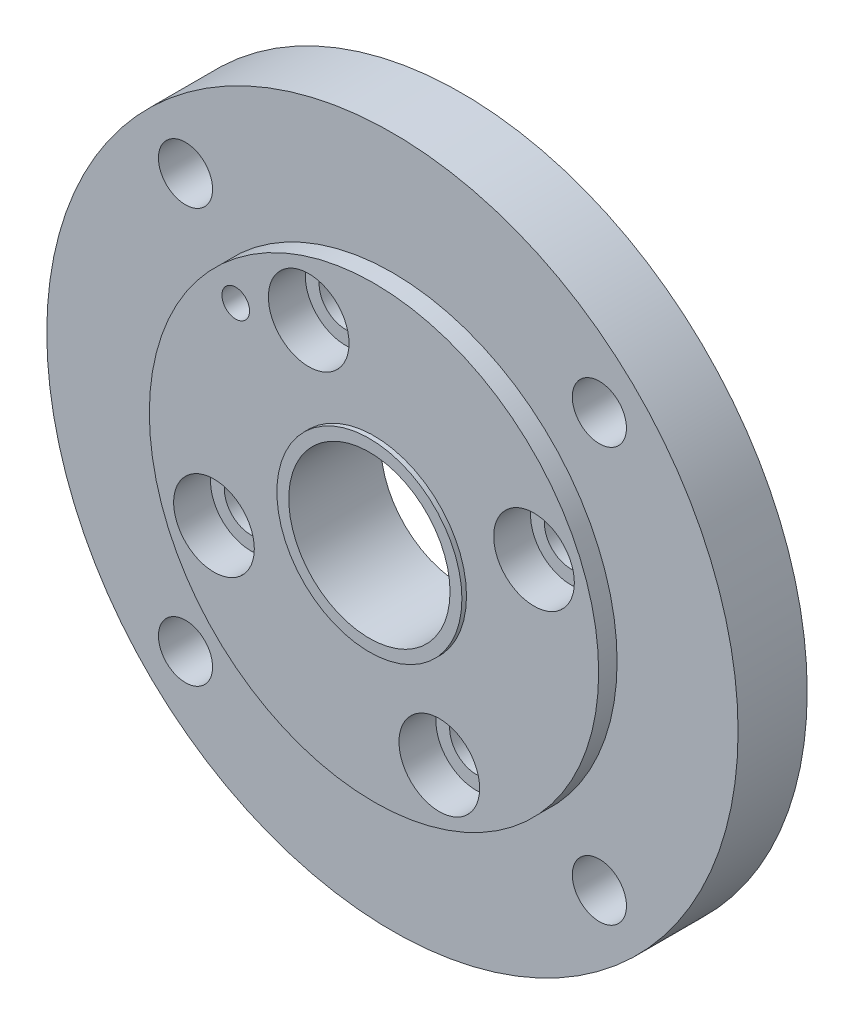
ISO-10303-21;
HEADER;
FILE_DESCRIPTION(('STEP AP214'),'2;1');
FILE_NAME('part.step','',(''),(''),'','','');
FILE_SCHEMA(('AUTOMOTIVE_DESIGN { 1 0 10303 214 1 1 1 1 }'));
ENDSEC;
DATA;
#1=APPLICATION_CONTEXT('core data for automotive mechanical design processes');
#2=APPLICATION_PROTOCOL_DEFINITION('international standard','automotive_design',2000,#1);
#3=PRODUCT_CONTEXT('',#1,'mechanical');
#4=PRODUCT('Part','Part','',(#3));
#5=PRODUCT_RELATED_PRODUCT_CATEGORY('part','',(#4));
#6=PRODUCT_DEFINITION_FORMATION('','',#4);
#7=PRODUCT_DEFINITION_CONTEXT('part definition',#1,'design');
#8=PRODUCT_DEFINITION('design','',#6,#7);
#9=PRODUCT_DEFINITION_SHAPE('','',#8);
#10=(LENGTH_UNIT() NAMED_UNIT(*) SI_UNIT(.MILLI.,.METRE.));
#11=(NAMED_UNIT(*) PLANE_ANGLE_UNIT() SI_UNIT($,.RADIAN.));
#12=(NAMED_UNIT(*) SI_UNIT($,.STERADIAN.) SOLID_ANGLE_UNIT());
#13=UNCERTAINTY_MEASURE_WITH_UNIT(LENGTH_MEASURE(1.E-05),#10,'distance_accuracy_value','');
#14=(GEOMETRIC_REPRESENTATION_CONTEXT(3) GLOBAL_UNCERTAINTY_ASSIGNED_CONTEXT((#13)) GLOBAL_UNIT_ASSIGNED_CONTEXT((#10,
#11,#12)) REPRESENTATION_CONTEXT('',''));
#15=CARTESIAN_POINT('',(0.,0.,0.));
#16=DIRECTION('',(0.,0.,1.));
#17=DIRECTION('',(1.,0.,0.));
#18=AXIS2_PLACEMENT_3D('',#15,#16,#17);
#19=CARTESIAN_POINT('',(0.,0.,30.));
#20=DIRECTION('',(0.,0.,-1.));
#21=DIRECTION('',(-1.,0.,0.));
#22=AXIS2_PLACEMENT_3D('',#19,#20,#21);
#23=CYLINDRICAL_SURFACE('',#22,150.);
#24=CARTESIAN_POINT('',(0.,0.,30.));
#25=DIRECTION('',(0.,0.,1.));
#26=DIRECTION('',(1.,0.,0.));
#27=AXIS2_PLACEMENT_3D('',#24,#25,#26);
#28=CIRCLE('',#27,150.);
#29=CARTESIAN_POINT('',(150.,0.,30.));
#30=VERTEX_POINT('',#29);
#31=EDGE_CURVE('E54',#30,#30,#28,.T.);
#32=ORIENTED_EDGE('',*,*,#31,.F.);
#33=EDGE_LOOP('',(#32));
#34=FACE_BOUND('',#33,.T.);
#35=CARTESIAN_POINT('',(0.,0.,0.));
#36=DIRECTION('',(0.,0.,1.));
#37=DIRECTION('',(1.,0.,0.));
#38=AXIS2_PLACEMENT_3D('',#35,#36,#37);
#39=CIRCLE('',#38,150.);
#40=CARTESIAN_POINT('',(150.,0.,0.));
#41=VERTEX_POINT('',#40);
#42=EDGE_CURVE('E65',#41,#41,#39,.T.);
#43=ORIENTED_EDGE('',*,*,#42,.T.);
#44=EDGE_LOOP('',(#43));
#45=FACE_BOUND('',#44,.T.);
#46=ADVANCED_FACE('F43',(#34,#45),#23,.T.);
#47=CARTESIAN_POINT('',(0.,0.,30.));
#48=DIRECTION('',(0.,0.,1.));
#49=DIRECTION('',(1.,0.,0.));
#50=AXIS2_PLACEMENT_3D('',#47,#48,#49);
#51=PLANE('',#50);
#52=CARTESIAN_POINT('',(-89.8025612106864,-89.8025612106967,30.));
#53=DIRECTION('',(0.,0.,1.));
#54=DIRECTION('',(1.,0.,0.));
#55=AXIS2_PLACEMENT_3D('',#52,#53,#54);
#56=CIRCLE('',#55,11.7500000000037);
#57=CARTESIAN_POINT('',(-78.0525612106827,-89.8025612106967,30.));
#58=VERTEX_POINT('',#57);
#59=EDGE_CURVE('E118',#58,#58,#56,.T.);
#60=ORIENTED_EDGE('',*,*,#59,.F.);
#61=EDGE_LOOP('',(#60));
#62=FACE_BOUND('',#61,.T.);
#63=CARTESIAN_POINT('',(89.8025612106966,-89.8025612106914,30.));
#64=DIRECTION('',(0.,0.,1.));
#65=DIRECTION('',(1.,0.,0.));
#66=AXIS2_PLACEMENT_3D('',#63,#64,#65);
#67=CIRCLE('',#66,11.7499999999988);
#68=CARTESIAN_POINT('',(101.552561210695,-89.8025612106914,30.));
#69=VERTEX_POINT('',#68);
#70=EDGE_CURVE('E120',#69,#69,#67,.T.);
#71=ORIENTED_EDGE('',*,*,#70,.F.);
#72=EDGE_LOOP('',(#71));
#73=FACE_BOUND('',#72,.T.);
#74=CARTESIAN_POINT('',(89.8025612106914,89.8025612106917,30.));
#75=DIRECTION('',(0.,0.,1.));
#76=DIRECTION('',(1.,0.,0.));
#77=AXIS2_PLACEMENT_3D('',#74,#75,#76);
#78=CIRCLE('',#77,11.75);
#79=CARTESIAN_POINT('',(101.552561210691,89.8025612106917,30.));
#80=VERTEX_POINT('',#79);
#81=EDGE_CURVE('E113',#80,#80,#78,.T.);
#82=ORIENTED_EDGE('',*,*,#81,.F.);
#83=EDGE_LOOP('',(#82));
#84=FACE_BOUND('',#83,.T.);
#85=CARTESIAN_POINT('',(-89.8025612106917,89.8025612106864,30.));
#86=DIRECTION('',(0.,0.,1.));
#87=DIRECTION('',(1.,0.,0.));
#88=AXIS2_PLACEMENT_3D('',#85,#86,#87);
#89=CIRCLE('',#88,11.7500000000053);
#90=CARTESIAN_POINT('',(-78.0525612106864,89.8025612106864,30.));
#91=VERTEX_POINT('',#90);
#92=EDGE_CURVE('E75',#91,#91,#89,.T.);
#93=ORIENTED_EDGE('',*,*,#92,.F.);
#94=EDGE_LOOP('',(#93));
#95=FACE_BOUND('',#94,.T.);
#96=CARTESIAN_POINT('',(0.,0.,30.));
#97=DIRECTION('',(0.,0.,1.));
#98=DIRECTION('',(1.,0.,0.));
#99=AXIS2_PLACEMENT_3D('',#96,#97,#98);
#100=CIRCLE('',#99,97.5);
#101=CARTESIAN_POINT('',(97.5,0.,30.));
#102=VERTEX_POINT('',#101);
#103=EDGE_CURVE('E49',#102,#102,#100,.T.);
#104=ORIENTED_EDGE('',*,*,#103,.F.);
#105=EDGE_LOOP('',(#104));
#106=FACE_BOUND('',#105,.T.);
#107=ORIENTED_EDGE('',*,*,#31,.T.);
#108=EDGE_LOOP('',(#107));
#109=FACE_BOUND('',#108,.T.);
#110=ADVANCED_FACE('F148',(#62,#73,#84,#95,#106,#109),#51,.T.);
#111=CARTESIAN_POINT('',(0.,0.,0.));
#112=DIRECTION('',(0.,0.,1.));
#113=DIRECTION('',(1.,0.,0.));
#114=AXIS2_PLACEMENT_3D('',#111,#112,#113);
#115=PLANE('',#114);
#116=CARTESIAN_POINT('',(0.,0.,0.));
#117=DIRECTION('',(0.,0.,1.));
#118=DIRECTION('',(1.,0.,0.));
#119=AXIS2_PLACEMENT_3D('',#116,#117,#118);
#120=CIRCLE('',#119,35.);
#121=CARTESIAN_POINT('',(35.,0.,0.));
#122=VERTEX_POINT('',#121);
#123=EDGE_CURVE('E170',#122,#122,#120,.T.);
#124=ORIENTED_EDGE('',*,*,#123,.T.);
#125=EDGE_LOOP('',(#124));
#126=FACE_BOUND('',#125,.T.);
#127=CARTESIAN_POINT('',(-28.3380590113851,69.4402938607496,0.));
#128=DIRECTION('',(0.,0.,1.));
#129=DIRECTION('',(1.,0.,0.));
#130=AXIS2_PLACEMENT_3D('',#127,#128,#129);
#131=CIRCLE('',#130,11.5);
#132=CARTESIAN_POINT('',(-16.8380590113851,69.4402938607496,0.));
#133=VERTEX_POINT('',#132);
#134=EDGE_CURVE('E46',#133,#133,#131,.T.);
#135=ORIENTED_EDGE('',*,*,#134,.T.);
#136=EDGE_LOOP('',(#135));
#137=FACE_BOUND('',#136,.T.);
#138=CARTESIAN_POINT('',(69.4402938607507,28.3380590113878,0.));
#139=DIRECTION('',(0.,0.,1.));
#140=DIRECTION('',(1.,0.,0.));
#141=AXIS2_PLACEMENT_3D('',#138,#139,#140);
#142=CIRCLE('',#141,11.5000000000026);
#143=CARTESIAN_POINT('',(80.9402938607533,28.3380590113878,0.));
#144=VERTEX_POINT('',#143);
#145=EDGE_CURVE('E78',#144,#144,#142,.T.);
#146=ORIENTED_EDGE('',*,*,#145,.T.);
#147=EDGE_LOOP('',(#146));
#148=FACE_BOUND('',#147,.T.);
#149=CARTESIAN_POINT('',(28.338059011389,-69.440293860748,0.));
#150=DIRECTION('',(0.,0.,1.));
#151=DIRECTION('',(1.,0.,0.));
#152=AXIS2_PLACEMENT_3D('',#149,#150,#151);
#153=CIRCLE('',#152,11.5000000000047);
#154=CARTESIAN_POINT('',(39.8380590113937,-69.440293860748,0.));
#155=VERTEX_POINT('',#154);
#156=EDGE_CURVE('E79',#155,#155,#153,.T.);
#157=ORIENTED_EDGE('',*,*,#156,.T.);
#158=EDGE_LOOP('',(#157));
#159=FACE_BOUND('',#158,.T.);
#160=CARTESIAN_POINT('',(-69.4402938607468,-28.3380590113863,0.));
#161=DIRECTION('',(0.,0.,1.));
#162=DIRECTION('',(1.,0.,0.));
#163=AXIS2_PLACEMENT_3D('',#160,#161,#162);
#164=CIRCLE('',#163,11.5000000000027);
#165=CARTESIAN_POINT('',(-57.9402938607441,-28.3380590113863,0.));
#166=VERTEX_POINT('',#165);
#167=EDGE_CURVE('E74',#166,#166,#164,.T.);
#168=ORIENTED_EDGE('',*,*,#167,.T.);
#169=EDGE_LOOP('',(#168));
#170=FACE_BOUND('',#169,.T.);
#171=CARTESIAN_POINT('',(-60.,60.,0.));
#172=DIRECTION('',(0.,0.,1.));
#173=DIRECTION('',(1.,0.,0.));
#174=AXIS2_PLACEMENT_3D('',#171,#172,#173);
#175=CIRCLE('',#174,6.);
#176=CARTESIAN_POINT('',(-54.,60.,0.));
#177=VERTEX_POINT('',#176);
#178=EDGE_CURVE('E110',#177,#177,#175,.T.);
#179=ORIENTED_EDGE('',*,*,#178,.T.);
#180=EDGE_LOOP('',(#179));
#181=FACE_BOUND('',#180,.T.);
#182=CARTESIAN_POINT('',(-89.8025612106864,-89.8025612106967,0.));
#183=DIRECTION('',(0.,0.,1.));
#184=DIRECTION('',(1.,0.,0.));
#185=AXIS2_PLACEMENT_3D('',#182,#183,#184);
#186=CIRCLE('',#185,11.7500000000037);
#187=CARTESIAN_POINT('',(-78.0525612106827,-89.8025612106967,0.));
#188=VERTEX_POINT('',#187);
#189=EDGE_CURVE('E102',#188,#188,#186,.T.);
#190=ORIENTED_EDGE('',*,*,#189,.T.);
#191=EDGE_LOOP('',(#190));
#192=FACE_BOUND('',#191,.T.);
#193=CARTESIAN_POINT('',(89.8025612106966,-89.8025612106914,0.));
#194=DIRECTION('',(0.,0.,1.));
#195=DIRECTION('',(1.,0.,0.));
#196=AXIS2_PLACEMENT_3D('',#193,#194,#195);
#197=CIRCLE('',#196,11.7499999999988);
#198=CARTESIAN_POINT('',(101.552561210695,-89.8025612106914,0.));
#199=VERTEX_POINT('',#198);
#200=EDGE_CURVE('E101',#199,#199,#197,.T.);
#201=ORIENTED_EDGE('',*,*,#200,.T.);
#202=EDGE_LOOP('',(#201));
#203=FACE_BOUND('',#202,.T.);
#204=CARTESIAN_POINT('',(89.8025612106914,89.8025612106917,0.));
#205=DIRECTION('',(0.,0.,1.));
#206=DIRECTION('',(1.,0.,0.));
#207=AXIS2_PLACEMENT_3D('',#204,#205,#206);
#208=CIRCLE('',#207,11.75);
#209=CARTESIAN_POINT('',(101.552561210691,89.8025612106917,0.));
#210=VERTEX_POINT('',#209);
#211=EDGE_CURVE('E98',#210,#210,#208,.T.);
#212=ORIENTED_EDGE('',*,*,#211,.T.);
#213=EDGE_LOOP('',(#212));
#214=FACE_BOUND('',#213,.T.);
#215=CARTESIAN_POINT('',(-89.8025612106917,89.8025612106864,0.));
#216=DIRECTION('',(0.,0.,1.));
#217=DIRECTION('',(1.,0.,0.));
#218=AXIS2_PLACEMENT_3D('',#215,#216,#217);
#219=CIRCLE('',#218,11.7500000000053);
#220=CARTESIAN_POINT('',(-78.0525612106864,89.8025612106864,0.));
#221=VERTEX_POINT('',#220);
#222=EDGE_CURVE('E71',#221,#221,#219,.T.);
#223=ORIENTED_EDGE('',*,*,#222,.T.);
#224=EDGE_LOOP('',(#223));
#225=FACE_BOUND('',#224,.T.);
#226=ORIENTED_EDGE('',*,*,#42,.F.);
#227=EDGE_LOOP('',(#226));
#228=FACE_BOUND('',#227,.T.);
#229=ADVANCED_FACE('F147',(#126,#137,#148,#159,#170,#181,#192,#203,#214,#225,#228),#115,.F.);
#230=CARTESIAN_POINT('',(0.,0.,38.));
#231=DIRECTION('',(0.,0.,-1.));
#232=DIRECTION('',(-1.,0.,0.));
#233=AXIS2_PLACEMENT_3D('',#230,#231,#232);
#234=CYLINDRICAL_SURFACE('',#233,97.5);
#235=CARTESIAN_POINT('',(0.,0.,38.));
#236=DIRECTION('',(0.,0.,1.));
#237=DIRECTION('',(1.,0.,0.));
#238=AXIS2_PLACEMENT_3D('',#235,#236,#237);
#239=CIRCLE('',#238,97.5);
#240=CARTESIAN_POINT('',(97.5,0.,38.));
#241=VERTEX_POINT('',#240);
#242=EDGE_CURVE('E62',#241,#241,#239,.T.);
#243=ORIENTED_EDGE('',*,*,#242,.F.);
#244=EDGE_LOOP('',(#243));
#245=FACE_BOUND('',#244,.T.);
#246=ORIENTED_EDGE('',*,*,#103,.T.);
#247=EDGE_LOOP('',(#246));
#248=FACE_BOUND('',#247,.T.);
#249=ADVANCED_FACE('F142',(#245,#248),#234,.T.);
#250=CARTESIAN_POINT('',(0.,0.,38.));
#251=DIRECTION('',(0.,0.,1.));
#252=DIRECTION('',(1.,0.,0.));
#253=AXIS2_PLACEMENT_3D('',#250,#251,#252);
#254=PLANE('',#253);
#255=CARTESIAN_POINT('',(-69.4402938607468,-28.3380590113863,38.));
#256=DIRECTION('',(0.,0.,1.));
#257=DIRECTION('',(1.,0.,0.));
#258=AXIS2_PLACEMENT_3D('',#255,#256,#257);
#259=CIRCLE('',#258,17.5000000000027);
#260=CARTESIAN_POINT('',(-51.9402938607441,-28.3380590113863,38.));
#261=VERTEX_POINT('',#260);
#262=EDGE_CURVE('E280',#261,#261,#259,.T.);
#263=ORIENTED_EDGE('',*,*,#262,.F.);
#264=EDGE_LOOP('',(#263));
#265=FACE_BOUND('',#264,.T.);
#266=CARTESIAN_POINT('',(-28.3380590113851,69.4402938607496,38.));
#267=DIRECTION('',(0.,0.,1.));
#268=DIRECTION('',(1.,0.,0.));
#269=AXIS2_PLACEMENT_3D('',#266,#267,#268);
#270=CIRCLE('',#269,17.5);
#271=CARTESIAN_POINT('',(-10.8380590113851,69.4402938607496,38.));
#272=VERTEX_POINT('',#271);
#273=EDGE_CURVE('E285',#272,#272,#270,.T.);
#274=ORIENTED_EDGE('',*,*,#273,.F.);
#275=EDGE_LOOP('',(#274));
#276=FACE_BOUND('',#275,.T.);
#277=CARTESIAN_POINT('',(69.4402938607507,28.3380590113879,38.));
#278=DIRECTION('',(0.,0.,1.));
#279=DIRECTION('',(1.,0.,0.));
#280=AXIS2_PLACEMENT_3D('',#277,#278,#279);
#281=CIRCLE('',#280,17.5000000000026);
#282=CARTESIAN_POINT('',(86.9402938607533,28.3380590113879,38.));
#283=VERTEX_POINT('',#282);
#284=EDGE_CURVE('E94',#283,#283,#281,.T.);
#285=ORIENTED_EDGE('',*,*,#284,.F.);
#286=EDGE_LOOP('',(#285));
#287=FACE_BOUND('',#286,.T.);
#288=CARTESIAN_POINT('',(28.338059011389,-69.440293860748,38.));
#289=DIRECTION('',(0.,0.,1.));
#290=DIRECTION('',(1.,0.,0.));
#291=AXIS2_PLACEMENT_3D('',#288,#289,#290);
#292=CIRCLE('',#291,17.5000000000047);
#293=CARTESIAN_POINT('',(45.8380590113938,-69.440293860748,38.));
#294=VERTEX_POINT('',#293);
#295=EDGE_CURVE('E84',#294,#294,#292,.T.);
#296=ORIENTED_EDGE('',*,*,#295,.F.);
#297=EDGE_LOOP('',(#296));
#298=FACE_BOUND('',#297,.T.);
#299=CARTESIAN_POINT('',(-60.,60.,38.));
#300=DIRECTION('',(0.,0.,1.));
#301=DIRECTION('',(1.,0.,0.));
#302=AXIS2_PLACEMENT_3D('',#299,#300,#301);
#303=CIRCLE('',#302,6.);
#304=CARTESIAN_POINT('',(-54.,60.,38.));
#305=VERTEX_POINT('',#304);
#306=EDGE_CURVE('E68',#305,#305,#303,.T.);
#307=ORIENTED_EDGE('',*,*,#306,.F.);
#308=EDGE_LOOP('',(#307));
#309=FACE_BOUND('',#308,.T.);
#310=CARTESIAN_POINT('',(0.,0.,38.));
#311=DIRECTION('',(0.,0.,1.));
#312=DIRECTION('',(1.,0.,0.));
#313=AXIS2_PLACEMENT_3D('',#310,#311,#312);
#314=CIRCLE('',#313,40.15);
#315=CARTESIAN_POINT('',(40.15,0.,38.));
#316=VERTEX_POINT('',#315);
#317=EDGE_CURVE('E10',#316,#316,#314,.T.);
#318=ORIENTED_EDGE('',*,*,#317,.F.);
#319=EDGE_LOOP('',(#318));
#320=FACE_BOUND('',#319,.T.);
#321=ORIENTED_EDGE('',*,*,#242,.T.);
#322=EDGE_LOOP('',(#321));
#323=FACE_BOUND('',#322,.T.);
#324=ADVANCED_FACE('F132',(#265,#276,#287,#298,#309,#320,#323),#254,.T.);
#325=CARTESIAN_POINT('',(0.,0.,40.));
#326=DIRECTION('',(0.,0.,-1.));
#327=DIRECTION('',(-1.,0.,0.));
#328=AXIS2_PLACEMENT_3D('',#325,#326,#327);
#329=CYLINDRICAL_SURFACE('',#328,40.15);
#330=CARTESIAN_POINT('',(0.,0.,40.));
#331=DIRECTION('',(0.,0.,1.));
#332=DIRECTION('',(1.,0.,0.));
#333=AXIS2_PLACEMENT_3D('',#330,#331,#332);
#334=CIRCLE('',#333,40.15);
#335=CARTESIAN_POINT('',(40.15,0.,40.));
#336=VERTEX_POINT('',#335);
#337=EDGE_CURVE('E56',#336,#336,#334,.T.);
#338=ORIENTED_EDGE('',*,*,#337,.F.);
#339=EDGE_LOOP('',(#338));
#340=FACE_BOUND('',#339,.T.);
#341=ORIENTED_EDGE('',*,*,#317,.T.);
#342=EDGE_LOOP('',(#341));
#343=FACE_BOUND('',#342,.T.);
#344=ADVANCED_FACE('F129',(#340,#343),#329,.T.);
#345=CARTESIAN_POINT('',(0.,0.,40.));
#346=DIRECTION('',(0.,0.,1.));
#347=DIRECTION('',(1.,0.,0.));
#348=AXIS2_PLACEMENT_3D('',#345,#346,#347);
#349=PLANE('',#348);
#350=CARTESIAN_POINT('',(0.,0.,40.));
#351=DIRECTION('',(0.,0.,1.));
#352=DIRECTION('',(1.,0.,0.));
#353=AXIS2_PLACEMENT_3D('',#350,#351,#352);
#354=CIRCLE('',#353,35.);
#355=CARTESIAN_POINT('',(35.,0.,40.));
#356=VERTEX_POINT('',#355);
#357=EDGE_CURVE('E257',#356,#356,#354,.T.);
#358=ORIENTED_EDGE('',*,*,#357,.F.);
#359=EDGE_LOOP('',(#358));
#360=FACE_BOUND('',#359,.T.);
#361=ORIENTED_EDGE('',*,*,#337,.T.);
#362=EDGE_LOOP('',(#361));
#363=FACE_BOUND('',#362,.T.);
#364=ADVANCED_FACE('F130',(#360,#363),#349,.T.);
#365=CARTESIAN_POINT('',(-60.,60.,0.));
#366=DIRECTION('',(0.,0.,1.));
#367=DIRECTION('',(1.,0.,0.));
#368=AXIS2_PLACEMENT_3D('',#365,#366,#367);
#369=CYLINDRICAL_SURFACE('',#368,6.);
#370=ORIENTED_EDGE('',*,*,#306,.T.);
#371=EDGE_LOOP('',(#370));
#372=FACE_BOUND('',#371,.T.);
#373=ORIENTED_EDGE('',*,*,#178,.F.);
#374=EDGE_LOOP('',(#373));
#375=FACE_BOUND('',#374,.T.);
#376=ADVANCED_FACE('F137',(#372,#375),#369,.F.);
#377=CARTESIAN_POINT('',(-89.8025612106917,89.8025612106864,0.));
#378=DIRECTION('',(0.,0.,1.));
#379=DIRECTION('',(1.,0.,0.));
#380=AXIS2_PLACEMENT_3D('',#377,#378,#379);
#381=CYLINDRICAL_SURFACE('',#380,11.7500000000053);
#382=ORIENTED_EDGE('',*,*,#92,.T.);
#383=EDGE_LOOP('',(#382));
#384=FACE_BOUND('',#383,.T.);
#385=ORIENTED_EDGE('',*,*,#222,.F.);
#386=EDGE_LOOP('',(#385));
#387=FACE_BOUND('',#386,.T.);
#388=ADVANCED_FACE('F181',(#384,#387),#381,.F.);
#389=CARTESIAN_POINT('',(89.8025612106914,89.8025612106917,0.));
#390=DIRECTION('',(0.,0.,1.));
#391=DIRECTION('',(1.,0.,0.));
#392=AXIS2_PLACEMENT_3D('',#389,#390,#391);
#393=CYLINDRICAL_SURFACE('',#392,11.75);
#394=ORIENTED_EDGE('',*,*,#81,.T.);
#395=EDGE_LOOP('',(#394));
#396=FACE_BOUND('',#395,.T.);
#397=ORIENTED_EDGE('',*,*,#211,.F.);
#398=EDGE_LOOP('',(#397));
#399=FACE_BOUND('',#398,.T.);
#400=ADVANCED_FACE('F183',(#396,#399),#393,.F.);
#401=CARTESIAN_POINT('',(89.8025612106966,-89.8025612106914,0.));
#402=DIRECTION('',(0.,0.,1.));
#403=DIRECTION('',(1.,0.,0.));
#404=AXIS2_PLACEMENT_3D('',#401,#402,#403);
#405=CYLINDRICAL_SURFACE('',#404,11.7499999999988);
#406=ORIENTED_EDGE('',*,*,#70,.T.);
#407=EDGE_LOOP('',(#406));
#408=FACE_BOUND('',#407,.T.);
#409=ORIENTED_EDGE('',*,*,#200,.F.);
#410=EDGE_LOOP('',(#409));
#411=FACE_BOUND('',#410,.T.);
#412=ADVANCED_FACE('F195',(#408,#411),#405,.F.);
#413=CARTESIAN_POINT('',(-89.8025612106864,-89.8025612106967,0.));
#414=DIRECTION('',(0.,0.,1.));
#415=DIRECTION('',(1.,0.,0.));
#416=AXIS2_PLACEMENT_3D('',#413,#414,#415);
#417=CYLINDRICAL_SURFACE('',#416,11.7500000000037);
#418=ORIENTED_EDGE('',*,*,#59,.T.);
#419=EDGE_LOOP('',(#418));
#420=FACE_BOUND('',#419,.T.);
#421=ORIENTED_EDGE('',*,*,#189,.F.);
#422=EDGE_LOOP('',(#421));
#423=FACE_BOUND('',#422,.T.);
#424=ADVANCED_FACE('F196',(#420,#423),#417,.F.);
#425=CARTESIAN_POINT('',(28.338059011389,-69.440293860748,22.));
#426=DIRECTION('',(0.,0.,1.));
#427=DIRECTION('',(1.,0.,0.));
#428=AXIS2_PLACEMENT_3D('',#425,#426,#427);
#429=CYLINDRICAL_SURFACE('',#428,17.5000000000047);
#430=CARTESIAN_POINT('',(28.338059011389,-69.440293860748,22.));
#431=DIRECTION('',(0.,0.,1.));
#432=DIRECTION('',(1.,0.,0.));
#433=AXIS2_PLACEMENT_3D('',#430,#431,#432);
#434=CIRCLE('',#433,17.5000000000047);
#435=CARTESIAN_POINT('',(45.8380590113938,-69.440293860748,22.));
#436=VERTEX_POINT('',#435);
#437=EDGE_CURVE('E90',#436,#436,#434,.T.);
#438=ORIENTED_EDGE('',*,*,#437,.F.);
#439=EDGE_LOOP('',(#438));
#440=FACE_BOUND('',#439,.T.);
#441=ORIENTED_EDGE('',*,*,#295,.T.);
#442=EDGE_LOOP('',(#441));
#443=FACE_BOUND('',#442,.T.);
#444=ADVANCED_FACE('F203',(#440,#443),#429,.F.);
#445=CARTESIAN_POINT('',(0.,0.,22.));
#446=DIRECTION('',(0.,0.,1.));
#447=DIRECTION('',(1.,0.,0.));
#448=AXIS2_PLACEMENT_3D('',#445,#446,#447);
#449=PLANE('',#448);
#450=CARTESIAN_POINT('',(28.338059011389,-69.440293860748,22.));
#451=DIRECTION('',(0.,0.,1.));
#452=DIRECTION('',(1.,0.,0.));
#453=AXIS2_PLACEMENT_3D('',#450,#451,#452);
#454=CIRCLE('',#453,11.5000000000047);
#455=CARTESIAN_POINT('',(39.8380590113937,-69.440293860748,22.));
#456=VERTEX_POINT('',#455);
#457=EDGE_CURVE('E262',#456,#456,#454,.T.);
#458=ORIENTED_EDGE('',*,*,#457,.F.);
#459=EDGE_LOOP('',(#458));
#460=FACE_BOUND('',#459,.T.);
#461=ORIENTED_EDGE('',*,*,#437,.T.);
#462=EDGE_LOOP('',(#461));
#463=FACE_BOUND('',#462,.T.);
#464=ADVANCED_FACE('F210',(#460,#463),#449,.T.);
#465=CARTESIAN_POINT('',(69.4402938607507,28.3380590113879,22.));
#466=DIRECTION('',(0.,0.,1.));
#467=DIRECTION('',(1.,0.,0.));
#468=AXIS2_PLACEMENT_3D('',#465,#466,#467);
#469=CYLINDRICAL_SURFACE('',#468,17.5000000000026);
#470=CARTESIAN_POINT('',(69.4402938607507,28.3380590113879,22.));
#471=DIRECTION('',(0.,0.,1.));
#472=DIRECTION('',(1.,0.,0.));
#473=AXIS2_PLACEMENT_3D('',#470,#471,#472);
#474=CIRCLE('',#473,17.5000000000026);
#475=CARTESIAN_POINT('',(86.9402938607533,28.3380590113879,22.));
#476=VERTEX_POINT('',#475);
#477=EDGE_CURVE('E286',#476,#476,#474,.T.);
#478=ORIENTED_EDGE('',*,*,#477,.F.);
#479=EDGE_LOOP('',(#478));
#480=FACE_BOUND('',#479,.T.);
#481=ORIENTED_EDGE('',*,*,#284,.T.);
#482=EDGE_LOOP('',(#481));
#483=FACE_BOUND('',#482,.T.);
#484=ADVANCED_FACE('F211',(#480,#483),#469,.F.);
#485=CARTESIAN_POINT('',(0.,0.,22.));
#486=DIRECTION('',(0.,0.,1.));
#487=DIRECTION('',(1.,0.,0.));
#488=AXIS2_PLACEMENT_3D('',#485,#486,#487);
#489=PLANE('',#488);
#490=CARTESIAN_POINT('',(69.4402938607507,28.3380590113878,22.));
#491=DIRECTION('',(0.,0.,1.));
#492=DIRECTION('',(1.,0.,0.));
#493=AXIS2_PLACEMENT_3D('',#490,#491,#492);
#494=CIRCLE('',#493,11.5000000000026);
#495=CARTESIAN_POINT('',(80.9402938607533,28.3380590113878,22.));
#496=VERTEX_POINT('',#495);
#497=EDGE_CURVE('E269',#496,#496,#494,.T.);
#498=ORIENTED_EDGE('',*,*,#497,.F.);
#499=EDGE_LOOP('',(#498));
#500=FACE_BOUND('',#499,.T.);
#501=ORIENTED_EDGE('',*,*,#477,.T.);
#502=EDGE_LOOP('',(#501));
#503=FACE_BOUND('',#502,.T.);
#504=ADVANCED_FACE('F214',(#500,#503),#489,.T.);
#505=CARTESIAN_POINT('',(-28.3380590113851,69.4402938607496,22.));
#506=DIRECTION('',(0.,0.,1.));
#507=DIRECTION('',(1.,0.,0.));
#508=AXIS2_PLACEMENT_3D('',#505,#506,#507);
#509=CYLINDRICAL_SURFACE('',#508,17.5);
#510=CARTESIAN_POINT('',(-28.3380590113851,69.4402938607496,22.));
#511=DIRECTION('',(0.,0.,1.));
#512=DIRECTION('',(1.,0.,0.));
#513=AXIS2_PLACEMENT_3D('',#510,#511,#512);
#514=CIRCLE('',#513,17.5);
#515=CARTESIAN_POINT('',(-10.8380590113851,69.4402938607496,22.));
#516=VERTEX_POINT('',#515);
#517=EDGE_CURVE('E278',#516,#516,#514,.T.);
#518=ORIENTED_EDGE('',*,*,#517,.F.);
#519=EDGE_LOOP('',(#518));
#520=FACE_BOUND('',#519,.T.);
#521=ORIENTED_EDGE('',*,*,#273,.T.);
#522=EDGE_LOOP('',(#521));
#523=FACE_BOUND('',#522,.T.);
#524=ADVANCED_FACE('F218',(#520,#523),#509,.F.);
#525=CARTESIAN_POINT('',(0.,0.,22.));
#526=DIRECTION('',(0.,0.,1.));
#527=DIRECTION('',(1.,0.,0.));
#528=AXIS2_PLACEMENT_3D('',#525,#526,#527);
#529=PLANE('',#528);
#530=CARTESIAN_POINT('',(-28.3380590113851,69.4402938607496,22.));
#531=DIRECTION('',(0.,0.,1.));
#532=DIRECTION('',(1.,0.,0.));
#533=AXIS2_PLACEMENT_3D('',#530,#531,#532);
#534=CIRCLE('',#533,11.5);
#535=CARTESIAN_POINT('',(-16.8380590113851,69.4402938607496,22.));
#536=VERTEX_POINT('',#535);
#537=EDGE_CURVE('E80',#536,#536,#534,.T.);
#538=ORIENTED_EDGE('',*,*,#537,.F.);
#539=EDGE_LOOP('',(#538));
#540=FACE_BOUND('',#539,.T.);
#541=ORIENTED_EDGE('',*,*,#517,.T.);
#542=EDGE_LOOP('',(#541));
#543=FACE_BOUND('',#542,.T.);
#544=ADVANCED_FACE('F224',(#540,#543),#529,.T.);
#545=CARTESIAN_POINT('',(-69.4402938607468,-28.3380590113863,22.));
#546=DIRECTION('',(0.,0.,1.));
#547=DIRECTION('',(1.,0.,0.));
#548=AXIS2_PLACEMENT_3D('',#545,#546,#547);
#549=CYLINDRICAL_SURFACE('',#548,17.5000000000027);
#550=CARTESIAN_POINT('',(-69.4402938607468,-28.3380590113863,22.));
#551=DIRECTION('',(0.,0.,1.));
#552=DIRECTION('',(1.,0.,0.));
#553=AXIS2_PLACEMENT_3D('',#550,#551,#552);
#554=CIRCLE('',#553,17.5000000000027);
#555=CARTESIAN_POINT('',(-51.9402938607441,-28.3380590113863,22.));
#556=VERTEX_POINT('',#555);
#557=EDGE_CURVE('E109',#556,#556,#554,.T.);
#558=ORIENTED_EDGE('',*,*,#557,.F.);
#559=EDGE_LOOP('',(#558));
#560=FACE_BOUND('',#559,.T.);
#561=ORIENTED_EDGE('',*,*,#262,.T.);
#562=EDGE_LOOP('',(#561));
#563=FACE_BOUND('',#562,.T.);
#564=ADVANCED_FACE('F229',(#560,#563),#549,.F.);
#565=CARTESIAN_POINT('',(0.,0.,22.));
#566=DIRECTION('',(0.,0.,1.));
#567=DIRECTION('',(1.,0.,0.));
#568=AXIS2_PLACEMENT_3D('',#565,#566,#567);
#569=PLANE('',#568);
#570=CARTESIAN_POINT('',(-69.4402938607468,-28.3380590113863,22.));
#571=DIRECTION('',(0.,0.,1.));
#572=DIRECTION('',(1.,0.,0.));
#573=AXIS2_PLACEMENT_3D('',#570,#571,#572);
#574=CIRCLE('',#573,11.5000000000027);
#575=CARTESIAN_POINT('',(-57.9402938607441,-28.3380590113863,22.));
#576=VERTEX_POINT('',#575);
#577=EDGE_CURVE('E261',#576,#576,#574,.T.);
#578=ORIENTED_EDGE('',*,*,#577,.F.);
#579=EDGE_LOOP('',(#578));
#580=FACE_BOUND('',#579,.T.);
#581=ORIENTED_EDGE('',*,*,#557,.T.);
#582=EDGE_LOOP('',(#581));
#583=FACE_BOUND('',#582,.T.);
#584=ADVANCED_FACE('F231',(#580,#583),#569,.T.);
#585=CARTESIAN_POINT('',(-69.4402938607468,-28.3380590113863,-8.));
#586=DIRECTION('',(0.,0.,1.));
#587=DIRECTION('',(1.,0.,0.));
#588=AXIS2_PLACEMENT_3D('',#585,#586,#587);
#589=CYLINDRICAL_SURFACE('',#588,11.5000000000027);
#590=ORIENTED_EDGE('',*,*,#577,.T.);
#591=EDGE_LOOP('',(#590));
#592=FACE_BOUND('',#591,.T.);
#593=ORIENTED_EDGE('',*,*,#167,.F.);
#594=EDGE_LOOP('',(#593));
#595=FACE_BOUND('',#594,.T.);
#596=ADVANCED_FACE('F234',(#592,#595),#589,.F.);
#597=CARTESIAN_POINT('',(28.338059011389,-69.440293860748,-8.));
#598=DIRECTION('',(0.,0.,1.));
#599=DIRECTION('',(1.,0.,0.));
#600=AXIS2_PLACEMENT_3D('',#597,#598,#599);
#601=CYLINDRICAL_SURFACE('',#600,11.5000000000047);
#602=ORIENTED_EDGE('',*,*,#457,.T.);
#603=EDGE_LOOP('',(#602));
#604=FACE_BOUND('',#603,.T.);
#605=ORIENTED_EDGE('',*,*,#156,.F.);
#606=EDGE_LOOP('',(#605));
#607=FACE_BOUND('',#606,.T.);
#608=ADVANCED_FACE('F239',(#604,#607),#601,.F.);
#609=CARTESIAN_POINT('',(69.4402938607507,28.3380590113878,-8.));
#610=DIRECTION('',(0.,0.,1.));
#611=DIRECTION('',(1.,0.,0.));
#612=AXIS2_PLACEMENT_3D('',#609,#610,#611);
#613=CYLINDRICAL_SURFACE('',#612,11.5000000000026);
#614=ORIENTED_EDGE('',*,*,#497,.T.);
#615=EDGE_LOOP('',(#614));
#616=FACE_BOUND('',#615,.T.);
#617=ORIENTED_EDGE('',*,*,#145,.F.);
#618=EDGE_LOOP('',(#617));
#619=FACE_BOUND('',#618,.T.);
#620=ADVANCED_FACE('F245',(#616,#619),#613,.F.);
#621=CARTESIAN_POINT('',(-28.3380590113851,69.4402938607496,-8.));
#622=DIRECTION('',(0.,0.,1.));
#623=DIRECTION('',(1.,0.,0.));
#624=AXIS2_PLACEMENT_3D('',#621,#622,#623);
#625=CYLINDRICAL_SURFACE('',#624,11.5);
#626=ORIENTED_EDGE('',*,*,#537,.T.);
#627=EDGE_LOOP('',(#626));
#628=FACE_BOUND('',#627,.T.);
#629=ORIENTED_EDGE('',*,*,#134,.F.);
#630=EDGE_LOOP('',(#629));
#631=FACE_BOUND('',#630,.T.);
#632=ADVANCED_FACE('F250',(#628,#631),#625,.F.);
#633=CARTESIAN_POINT('',(0.,0.,-10.));
#634=DIRECTION('',(0.,0.,1.));
#635=DIRECTION('',(1.,0.,0.));
#636=AXIS2_PLACEMENT_3D('',#633,#634,#635);
#637=CYLINDRICAL_SURFACE('',#636,35.);
#638=ORIENTED_EDGE('',*,*,#357,.T.);
#639=EDGE_LOOP('',(#638));
#640=FACE_BOUND('',#639,.T.);
#641=ORIENTED_EDGE('',*,*,#123,.F.);
#642=EDGE_LOOP('',(#641));
#643=FACE_BOUND('',#642,.T.);
#644=ADVANCED_FACE('F253',(#640,#643),#637,.F.);
#645=CLOSED_SHELL('',(#46,#110,#229,#249,#324,#344,#364,#376,#388,#400,#412,#424,#444,#464,#484,
#504,#524,#544,#564,#584,#596,#608,#620,#632,#644));
#646=MANIFOLD_SOLID_BREP('B2',#645);
#647=ADVANCED_BREP_SHAPE_REPRESENTATION('',(#18,#646),#14);
#648=SHAPE_DEFINITION_REPRESENTATION(#9,#647);
ENDSEC;
END-ISO-10303-21;
